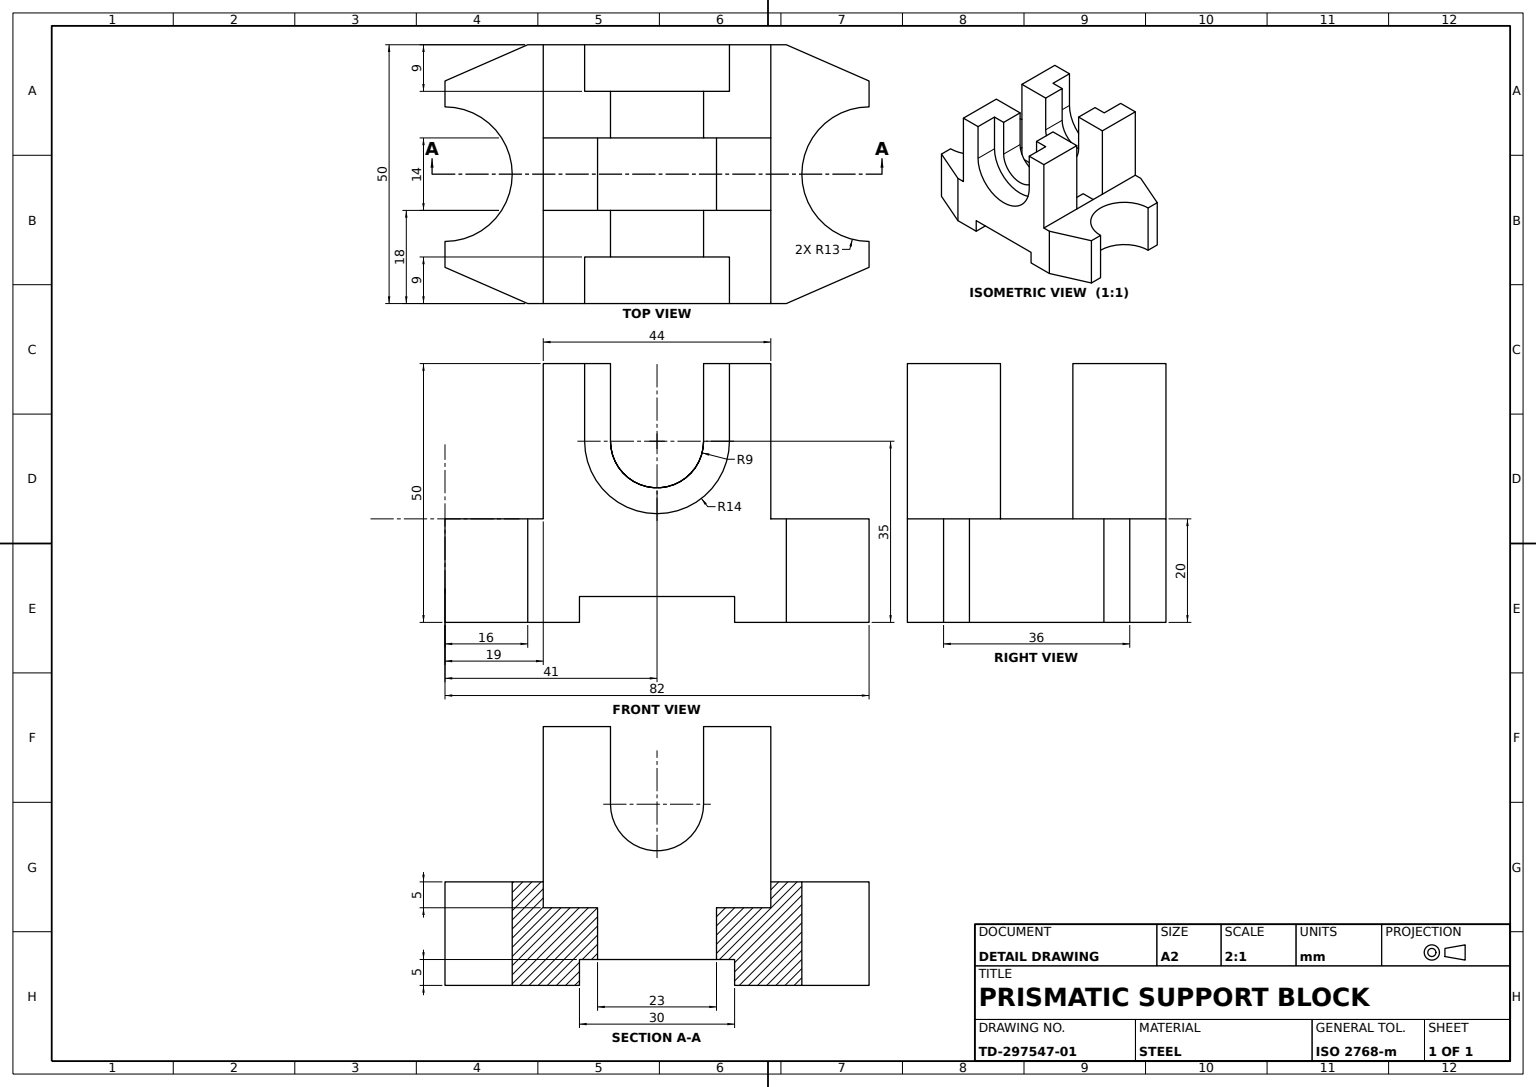
from build123d import *

# Parameters (mm, degrees)
BASE_BLOCK_DEPTH         = 20
UPRIGHTS_DEPTH           = 18
UPRIGHT_NOTCH_DEPTH      = 9
UNDERSIDE_SLOT_PROFILE_W = 30
UNDERSIDE_SLOT_PROFILE_H = 10
UNDERSIDE_SLOT_DEPTH     = 82.737384348
SADDLE_CUT_PROFILE_W     = 23
SADDLE_CUT_PROFILE_H     = 14
SADDLE_CUT_DEPTH         = 57.621550668
UPRIGHT_SLOT_PROFILE_W   = 44
UPRIGHT_SLOT_PROFILE_H   = 14
UPRIGHT_SLOT_CUT_DEPTH   = 5


with BuildPart() as part:
    # Base Block Profile → Base Block (new body)
    with BuildSketch(Plane(origin=(0, 0, 0), x_dir=(1, 0, 0), z_dir=(0, 1, 0))):
        with BuildLine():
            Line((-25, 25), (25, 25))
            Line((25, 25), (41, 18))
            Line((41, 18), (41, 13))
            ThreePointArc((41, 13), (28, 0), (41, -13))
            Line((41, -13), (41, -18))
            Line((41, -18), (25, -25))
            Line((25, -25), (-25, -25))
            Line((-25, -25), (-41, -18))
            Line((-41, -18), (-41, -13))
            ThreePointArc((-41, -13), (-28, 0), (-41, 13))
            Line((-41, 13), (-41, 18))
            Line((-41, 18), (-25, 25))
        make_face()
    extrude(amount=BASE_BLOCK_DEPTH)

    # Uprights Profile → Uprights (add)
    with BuildSketch(Plane.XY.offset(25)):
        with BuildLine():
            Line((-22, 20), (-22, 50))
            Line((-22, 50), (-9, 50))
            Line((-9, 50), (-9, 35))
            ThreePointArc((-9, 35), (0, 26), (9, 35))
            Line((9, 35), (9, 50))
            Line((9, 50), (22, 50))
            Line((22, 50), (22, 20))
            Line((22, 20), (-22, 20))
        make_face()
    uprights = extrude(amount=-UPRIGHTS_DEPTH)

    # Upright Notch Profile → Upright Notch (cut)
    with BuildSketch(Plane.XY.offset(25)):
        with BuildLine():
            Line((-14, 50), (14, 50))
            Line((14, 50), (14, 35))
            ThreePointArc((14, 35), (0, 21), (-14, 35))
            Line((-14, 35), (-14, 50))
        make_face()
    upright_notch = extrude(amount=-UPRIGHT_NOTCH_DEPTH, mode=Mode.SUBTRACT)

    # Upright Notch Mirror: Uprights, Upright Notch across plane
    add(uprights.mirror(Plane.XY))
    add(upright_notch.mirror(Plane.XY), mode=Mode.SUBTRACT)

    # Underside Slot Profile → Underside Slot (cut, through all)
    with BuildSketch(Plane.XY.offset(25)):
        Rectangle(UNDERSIDE_SLOT_PROFILE_W, UNDERSIDE_SLOT_PROFILE_H)
    extrude(amount=-UNDERSIDE_SLOT_DEPTH, mode=Mode.SUBTRACT)

    # Saddle Cut Profile → Saddle Cut (cut, through all)
    with BuildSketch(Plane(origin=(0, 20, 0), x_dir=(1, 0, 0), z_dir=(0, 1, 0))):
        Rectangle(SADDLE_CUT_PROFILE_W, SADDLE_CUT_PROFILE_H)
    extrude(amount=-SADDLE_CUT_DEPTH, mode=Mode.SUBTRACT)

    # Upright Slot Profile → Upright Slot Cut (cut)
    with BuildSketch(Plane(origin=(0, 20, 0), x_dir=(1, 0, 0), z_dir=(0, 1, 0))):
        Rectangle(UPRIGHT_SLOT_PROFILE_W, UPRIGHT_SLOT_PROFILE_H)
    extrude(amount=-UPRIGHT_SLOT_CUT_DEPTH, mode=Mode.SUBTRACT)


solid = part.part
